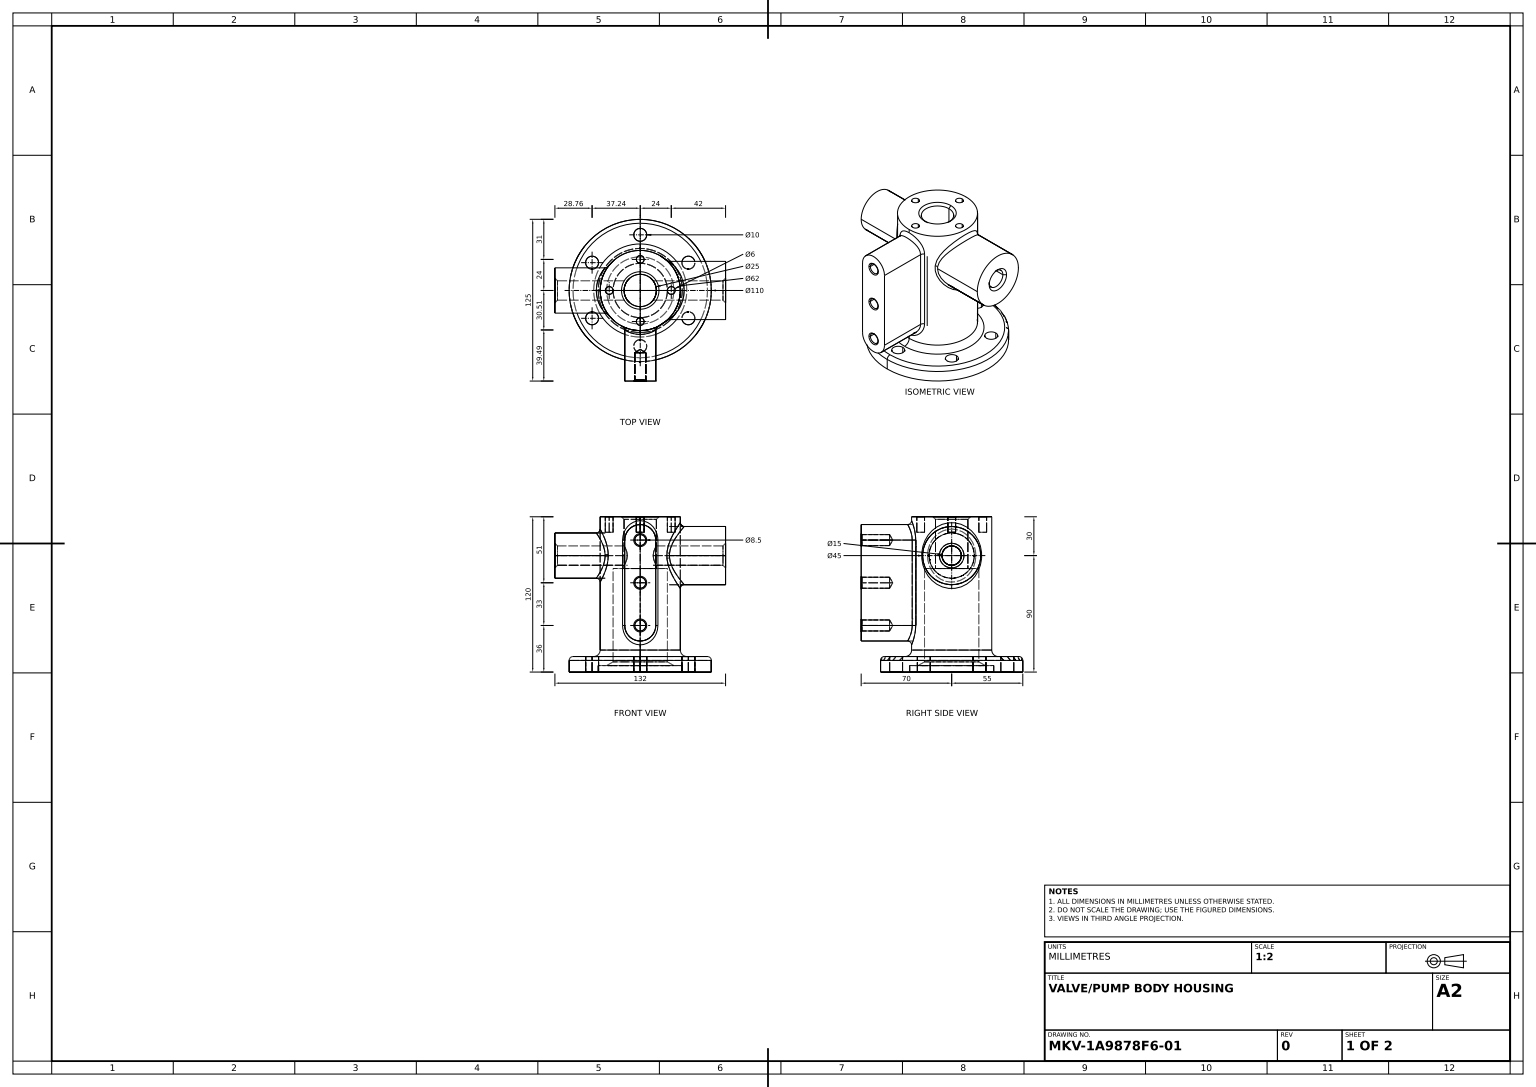
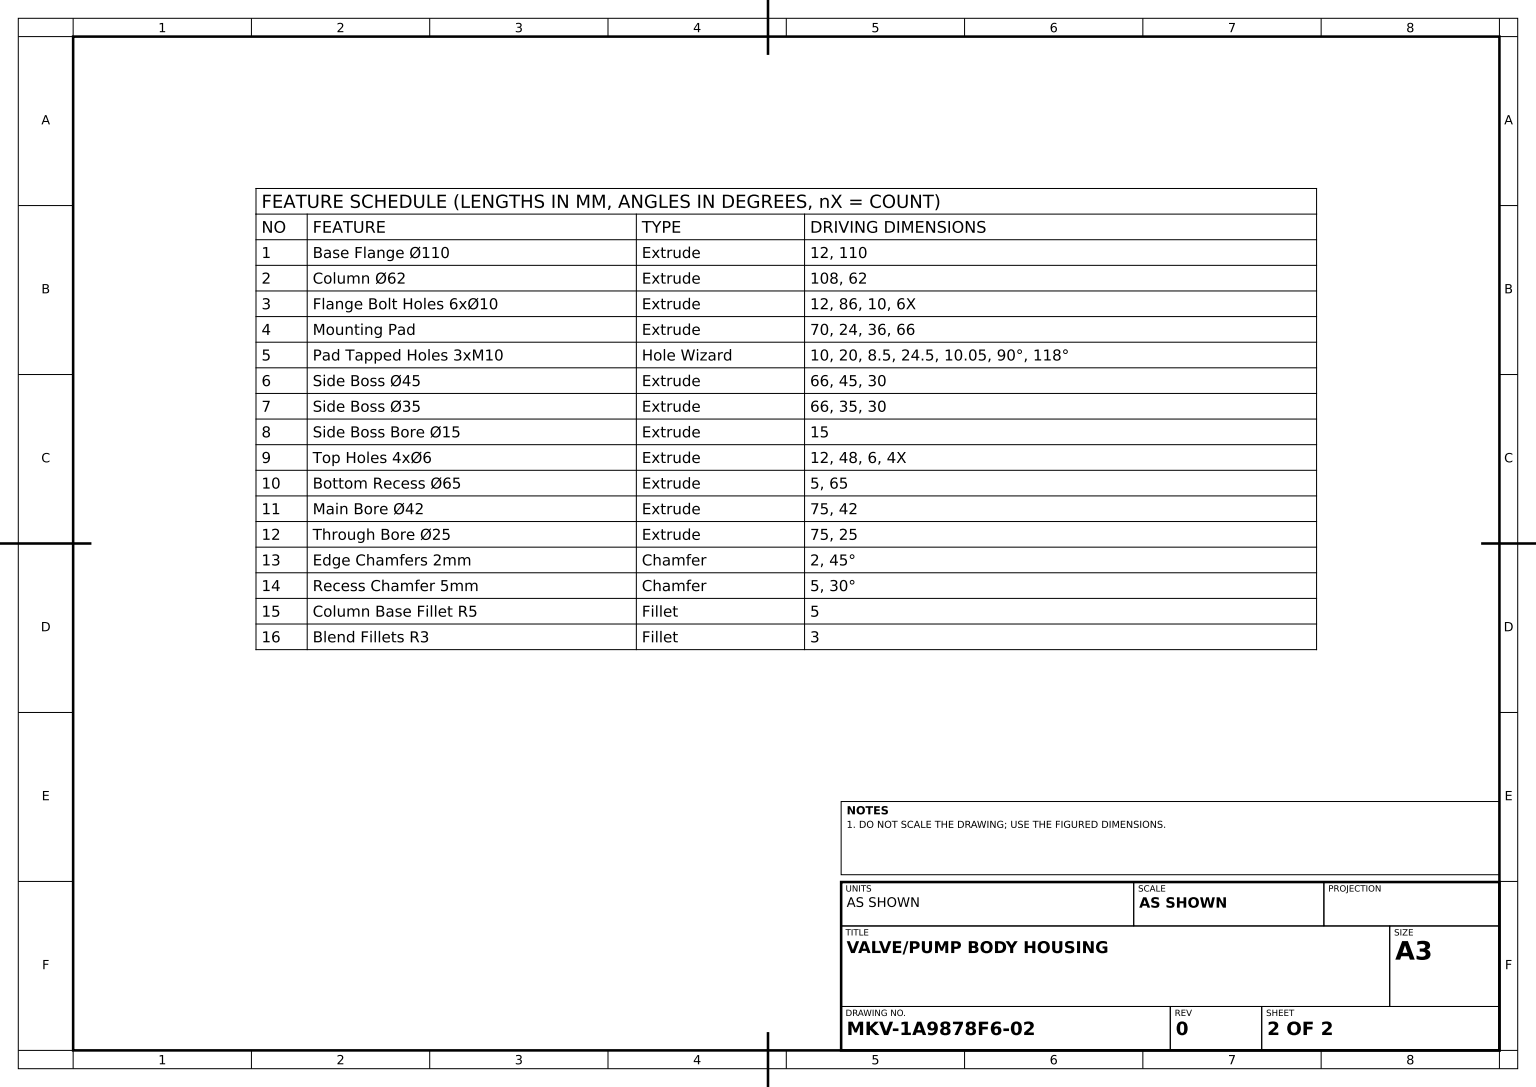
SolidWorks part; units mm, degrees
material "Plain Carbon Steel"
ref_plane "Front Plane" through (0, 0, 0) normal (0, 0, 1) x (1, 0, 0)
ref_plane "Top Plane" through (0, 0, 0) normal (0, 1, 0) x (1, 0, 0)
ref_plane "Right Plane" through (0, 0, 0) normal (1, 0, 0) x (0, 0, -1)
sketch "Base Flange Sketch" plane through (0, 0, 0) normal (0, 1, 0) x (1, 0, 0)
  circle A0 centre (0, 0) radius 55
  dimension "D1" = 110
extrude "Base Flange Ø110" add sketch "Base Flange Sketch" along normal blind 12
sketch "Column Sketch" plane through (0, 12, 0) normal (0, 1, 0) x (1, 0, 0)
  circle A0 centre (0, 0) radius 31
  dimension "D1" = 62
extrude "Column Ø62" add sketch "Column Sketch" along normal blind 108
sketch "Flange Bolt Holes Sketch" plane through (0, 12, 0) normal (0, 1, 0) x (1, 0, 0)
  circle A0 centre (0, 0) radius 43 construction
  circle A1 centre (0, 43) radius 5
  circle A2 centre (37.2391, 21.5) radius 5
  circle A3 centre (37.2391, -21.5) radius 5
  circle A4 centre (0, -43) radius 5
  circle A5 centre (-37.2391, -21.5) radius 5
  circle A6 centre (-37.2391, 21.5) radius 5
  dimension "D1" = 86
  dimension "D2" = 10
  dimension "D3" = 6
extrude "Flange Bolt Holes 6xØ10" cut sketch "Flange Bolt Holes Sketch" against normal blind 12
ref_plane "Plane1" through (0, 0, 70) normal (0, 0, 1) x (1, 0, 0)
sketch "Mounting Pad Sketch" plane through (0, 0, 70) normal (0, 0, 1) x (1, 0, 0)
  line L1 (-55, 0) -> (55, 0) construction
  line L2 (-12, 102) -> (-12, 36)
  line L3 (12, 102) -> (12, 36)
  arc A0 (12, 102) -> (-12, 102) centre (0, 102) ccw
  arc A1 (-12, 36) -> (12, 36) centre (0, 36) ccw
  dimension "D1" = 24
  dimension "D2" = 36
  dimension "D3" = 66
extrude "Mounting Pad" add sketch "Mounting Pad Sketch" against normal up to next
sketch "Pad Tapped Holes Positions" plane through (0, 0, 70) normal (0, 0, 1) x (1, 0, 0)
  point P0 (0, 102)
  point P1 (0, 36)
  point P3 (0, 69)
  dimension "D1" = 33
hole_wizard "Pad Tapped Holes 3xM10" positions "Sketch9" profile "Sketch10" tap size "M10" standard "ISO"
sketch "Sketch9" plane through (0, 0, 70) normal (0, 0, 1) x (1, 0, 0)
  point P0 (0, 102)
  point P3 (0, 69)
  point P6 (0, 36)
sketch "Sketch10" plane through (0, 102, 70) normal (1, 0, 0) x (0, -1, 0)
  line L0 (0, 0) -> (0, 24.5)
  line L1 (0, 24.5) -> (4.25, 21.9463)
  line L2 (4.25, 21.9463) -> (4.25, 0.775)
  line L3 (4.25, 0.775) -> (5.025, 0)
  line L5 (5.025, 0) -> (0, 0)
  line L6 (-4.25, 0.775) -> (-5.025, 0) construction
  line L10 (0, 24.5) -> (-4.25, 21.9463) construction
  line L11 (0, -6.35) -> (0, 107.95) construction
  dimension "Tap Drill Dia." = 8.5
  dimension "Tap Drill Depth" = 24.5
  dimension "Near C'Sink Dia." = 10.05
  dimension "Near C'Sink Angle" = 90
  dimension "Drill Angle" = 118
cosmetic thread "Hole Thread4" parameters "D1"=20, "D2"=10
cosmetic thread "Hole Thread5" parameters "D1"=20, "D2"=10
cosmetic thread "Hole Thread6" parameters "D1"=20, "D2"=10
ref_plane "Plane2" through (66, 0, 0) normal (1, 0, 0) x (0, 0, -1)
sketch "Side Boss Ø45 Sketch" plane through (66, 0, 0) normal (1, 0, 0) x (0, 0, -1)
  line L0 (31, 120) -> (-31, 120) construction
  circle A0 centre (0, 90) radius 22.5
  dimension "D1" = 45
  dimension "D2" = 30
extrude "Side Boss Ø45" add sketch "Side Boss Ø45 Sketch" against normal up to next
ref_plane "Plane3" through (-66, 0, 0) normal (1, 0, 0) x (0, 0, -1)
sketch "Side Boss Ø35 Sketch" plane through (-66, 0, 0) normal (1, 0, 0) x (0, 0, -1)
  line L0 (31, 120) -> (-31, 120) construction
  circle A0 centre (0, 90) radius 17.5
  dimension "D1" = 35
  dimension "D2" = 30
extrude "Side Boss Ø35" add sketch "Side Boss Ø35 Sketch" along normal up to next
sketch "Side Boss Bore Sketch" plane through (66, 0, 0) normal (1, 0, 0) x (0, 0, -1)
  circle A0 centre (0, 90) radius 7.5
  dimension "D1" = 15
extrude "Side Boss Bore Ø15" cut sketch "Side Boss Bore Sketch" against normal through all
sketch "Top Holes Sketch" plane through (0, 120, 0) normal (0, 1, 0) x (1, 0, 0)
  circle A0 centre (0, 0) radius 24 construction
  circle A1 centre (0, 24) radius 3
  circle A2 centre (24, 0) radius 3
  circle A3 centre (0, -24) radius 3
  circle A4 centre (-24, 0) radius 3
  dimension "D1" = 48
  dimension "D2" = 6
  dimension "D3" = 4
extrude "Top Holes 4xØ6" cut sketch "Top Holes Sketch" against normal blind 12
sketch "Bottom Recess Sketch" plane through (0, 0, 0) normal (0, -1, 0) x (1, 0, 0)
  circle A0 centre (0, 0) radius 32.5
  dimension "D1" = 65
extrude "Bottom Recess Ø65" cut sketch "Bottom Recess Sketch" against normal blind 5
sketch "Main Bore Sketch" plane through (0, 5, 0) normal (0, -1, 0) x (1, 0, 0)
  circle A0 centre (0, 0) radius 21
  dimension "D1" = 42
extrude "Main Bore Ø42" cut sketch "Main Bore Sketch" against normal blind 75
sketch "Through Bore Sketch" plane through (0, 80, 0) normal (0, -1, 0) x (1, 0, 0)
  circle A0 centre (0, 0) radius 12.5
  dimension "D1" = 25
extrude "Through Bore Ø25" cut sketch "Through Bore Sketch" against normal blind 75
chamfer "Edge Chamfers 2mm" distance 2 angle 45 3 edges at (66, 90, -7.5) (-66, 90, -7.5) (0, 120, 12.5)
chamfer "Recess Chamfer 5mm" distance 5 angle 30 1 edges at (0, 5, -21)
fillet "Column Base Fillet R5" radius 5 1 edges at (0, 12, 31)
fillet "Blend Fillets R3" radius 3 7 edges at (0.9723, 24.0395, 30.9847) (-12, 69, 28.5832) (-0.9723, 113.9605, 30.9847) (0, 12, 55) (-25.592, 89.553, -17.4943) (12, 69, 28.5832) (21.3583, 88.806, 22.4683)
